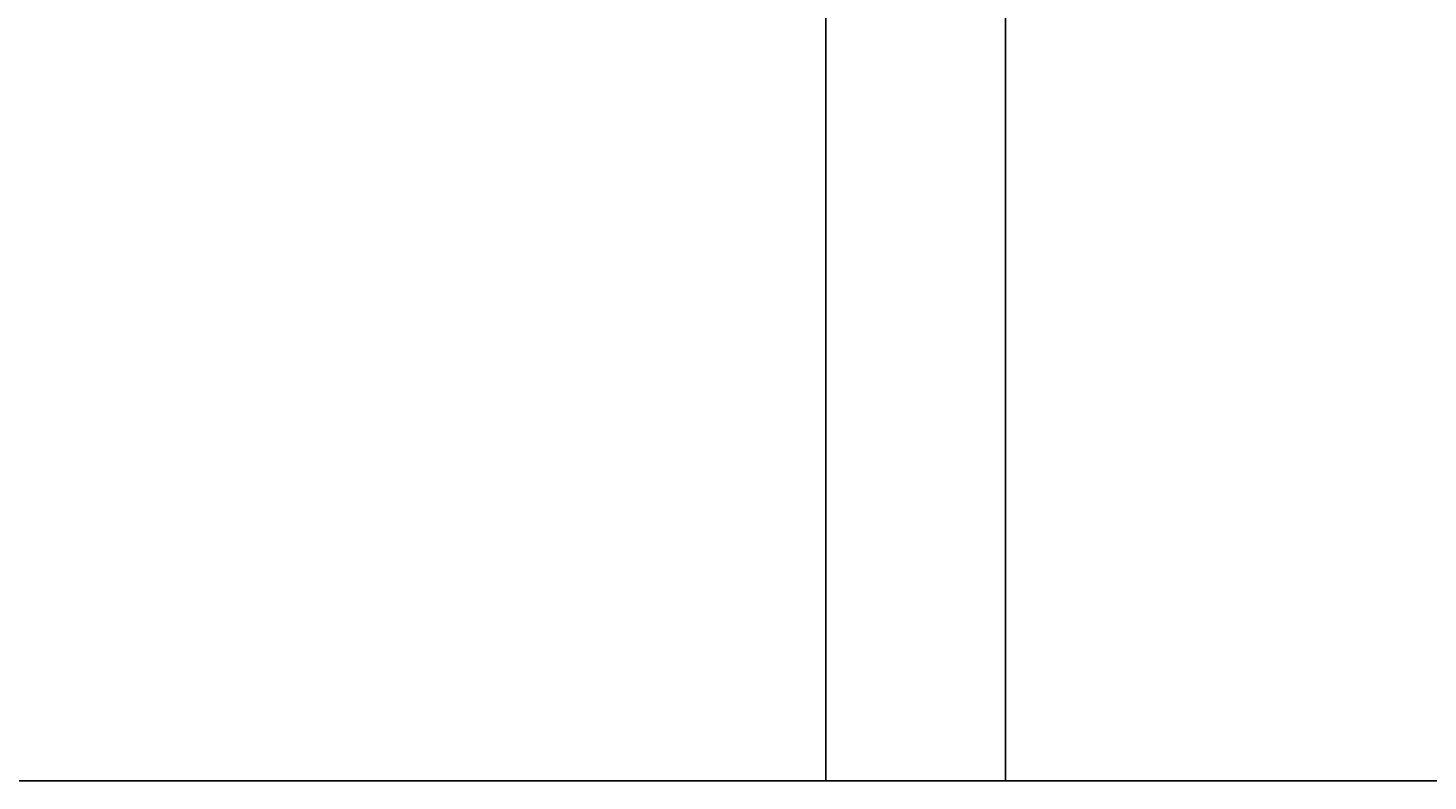
# Model space of a CAD drawing. Units: inches. Extents: x 35362 to 73946, y 43607 to 67532.
# Tile 15 of 134: x 46225 to 49302, y 43607 to 45263. Entities that reach past the tile are written whole.
import ezdxf

# ---------------------------------------------------------------- set-up
doc = ezdxf.new("R2010")
doc.units = ezdxf.units.IN
doc.header["$MEASUREMENT"] = 0
doc.layers.add('A-ANNO-DIMS', color=2, linetype='Continuous', lineweight=18)
doc.styles.get("Standard").update_dxf_attribs({"font": 'arial.ttf'})
doc.dimstyles.get("Standard").update_dxf_attribs({"dimtxt": 0.18, "dimasz": 0.18, "dimexe": 0.18, "dimexo": 0.0625, "dimgap": 0.09, "dimtad": 0, "dimtih": 1, "dimtoh": 1, "dimdec": 4, "dimzin": 0, "dimdsep": 46, "dimtxsty": 'Standard', "dimcen": 0.09, "dimadec": 0, "dimazin": 0, "dimtfac": 1, "dimtdec": 4, "dimtofl": 0, "dimtmove": 0, "dimatfit": 3, "dimfxl": 1, "dimtolj": 1, "dimtzin": 0, "dimarcsym": 0})

# ---------------------------------------------------------------- blocks, each defined once
blk = doc.blocks.new('*D5')
at = {"layer": 'A-ANNO-DIMS', "color": 0, "lineweight": -2, "transparency": 16777216}
for p, q in [((37121.9, 46919.3), (37121.9, 43606.7)), ((69871.5, 45449.8), (69871.5, 43606.7)), ((37122.1, 43606.9), (53496.3, 43606.9)), ((69871.3, 43606.9), (53497.2, 43606.9))]:
    blk.add_line(p, q, dxfattribs=at)
at = {"layer": 'A-ANNO-DIMS', "color": 0, "transparency": 16777216}
for points in [[(37122.1, 43606.9), (37122.1, 43606.8), (37121.9, 43606.9)], [(69871.3, 43606.9), (69871.3, 43606.8), (69871.5, 43606.9)]]:
    blk.add_solid(points, dxfattribs=at)
at = {"layer": 'Defpoints', "color": 0, "transparency": 16777216}
for p in [(37121.9, 46919.4), (69871.5, 45449.9), (69871.5, 43606.9)]:
    blk.add_point(p, dxfattribs=at)
at = {"layer": 'A-ANNO-DIMS', "color": 0, "transparency": 16777216, "insert": (53496.7, 43606.9), "char_height": 0.18, "attachment_point": 5}
blk.add_mtext('\\A1;32750', dxfattribs=at)
blk = doc.blocks.new('*D11')
at = {"layer": 'A-ANNO-DIMS', "color": 0, "lineweight": -2, "transparency": 16777216}
for p, q in [((47978.7, 56028.8), (47978.7, 43606.7)), ((53109.8, 56028.8), (53109.8, 43606.7)), ((47978.8, 43606.9), (50543.9, 43606.9)), ((53109.6, 43606.9), (50544.6, 43606.9))]:
    blk.add_line(p, q, dxfattribs=at)
at = {"layer": 'A-ANNO-DIMS', "color": 0, "transparency": 16777216}
for points in [[(47978.8, 43606.9), (47978.8, 43606.8), (47978.7, 43606.9)], [(53109.6, 43606.9), (53109.6, 43606.8), (53109.8, 43606.9)]]:
    blk.add_solid(points, dxfattribs=at)
at = {"layer": 'Defpoints', "color": 0, "transparency": 16777216}
for p in [(47978.7, 56028.8), (53109.8, 56028.8), (53109.8, 43606.9)]:
    blk.add_point(p, dxfattribs=at)
at = {"layer": 'A-ANNO-DIMS', "color": 0, "transparency": 16777216, "insert": (50544.2, 43606.9), "char_height": 0.18, "attachment_point": 5}
blk.add_mtext('\\A1;5131', dxfattribs=at)
blk = doc.blocks.new('*D13')
at = {"layer": 'A-ANNO-DIMS', "color": 0, "lineweight": -2, "transparency": 16777216}
for p, q in [((48373.5, 51694), (48373.5, 43606.7)), ((51029, 51694), (51029, 43606.7)), ((48373.7, 43606.9), (49700.8, 43606.9)), ((51028.9, 43606.9), (49701.7, 43606.9))]:
    blk.add_line(p, q, dxfattribs=at)
at = {"layer": 'A-ANNO-DIMS', "color": 0, "transparency": 16777216}
for points in [[(48373.7, 43606.9), (48373.7, 43606.8), (48373.5, 43606.9)], [(51028.9, 43606.9), (51028.9, 43606.8), (51029, 43606.9)]]:
    blk.add_solid(points, dxfattribs=at)
at = {"layer": 'Defpoints', "color": 0, "transparency": 16777216}
for p in [(48373.5, 51694.1), (51029, 51694.1), (51029, 43606.9)]:
    blk.add_point(p, dxfattribs=at)
at = {"layer": 'A-ANNO-DIMS', "color": 0, "transparency": 16777216, "insert": (49701.3, 43606.9), "char_height": 0.18, "attachment_point": 5}
blk.add_mtext('\\A1;2655.6', dxfattribs=at)
blk = doc.blocks.new('*D27')
at = {"layer": 'A-ANNO-DIMS', "color": 0, "lineweight": -2, "transparency": 16777216}
for p, q in [((47978.7, 56028.8), (47978.7, 43606.7)), ((48373.5, 53429), (48373.5, 43606.7)), ((47978.8, 43606.9), (48175.7, 43606.9)), ((48373.3, 43606.9), (48176.5, 43606.9))]:
    blk.add_line(p, q, dxfattribs=at)
at = {"layer": 'A-ANNO-DIMS', "color": 0, "transparency": 16777216}
for points in [[(47978.8, 43606.9), (47978.8, 43606.8), (47978.7, 43606.9)], [(48373.3, 43606.9), (48373.3, 43606.8), (48373.5, 43606.9)]]:
    blk.add_solid(points, dxfattribs=at)
at = {"layer": 'Defpoints', "color": 0, "transparency": 16777216}
for p in [(47978.7, 56028.8), (48373.5, 53429), (48373.5, 43606.9)]:
    blk.add_point(p, dxfattribs=at)
at = {"layer": 'A-ANNO-DIMS', "color": 0, "transparency": 16777216, "insert": (48176.1, 43606.9), "char_height": 0.18, "attachment_point": 5}
blk.add_mtext('\\A1;394.8', dxfattribs=at)

msp = doc.modelspace()

# ---------------------------------------------------------------- dimensions: what is measured, and where the dimension line sits
at = {"layer": 'A-ANNO-DIMS'}
for base, p1, p2, override, picture, middle in [((53109.76, 43606.859), (47978.665, 56028.836), (53109.76, 56028.836), {"dimdec": 0, "dimlfac": 1, "dimrnd": 0, "dimzin": 0, "dimdsep": 46, "dimlunit": 2}, '*D11', (50544.212, 43606.859)), ((48373.492, 43606.859), (47978.665, 56028.836), (48373.492, 53429.019), {"dimdec": 1, "dimlfac": 1, "dimrnd": 0, "dimzin": 0, "dimdsep": 46, "dimlunit": 2}, '*D27', (48176.078, 43606.859)), ((51029.043, 43606.859), (48373.492, 51694.087), (51029.043, 51694.087), {"dimdec": 1, "dimlfac": 1, "dimrnd": 0, "dimzin": 0, "dimdsep": 46, "dimlunit": 2}, '*D13', (49701.267, 43606.859)), ((69871.496, 43606.859), (37121.949, 46919.381), (69871.496, 45449.894), {"dimdec": 0, "dimlfac": 1, "dimrnd": 0, "dimzin": 0, "dimdsep": 46, "dimlunit": 2}, '*D5', (53496.723, 43606.859))]:
    dim = msp.add_linear_dim(base=base, p1=p1, p2=p2, dimstyle='Standard', override=override, dxfattribs=at)
    dim.commit()
    dim.dimension.update_dxf_attribs({"geometry": picture, "text_midpoint": middle})

doc.saveas('drawing.dxf')
